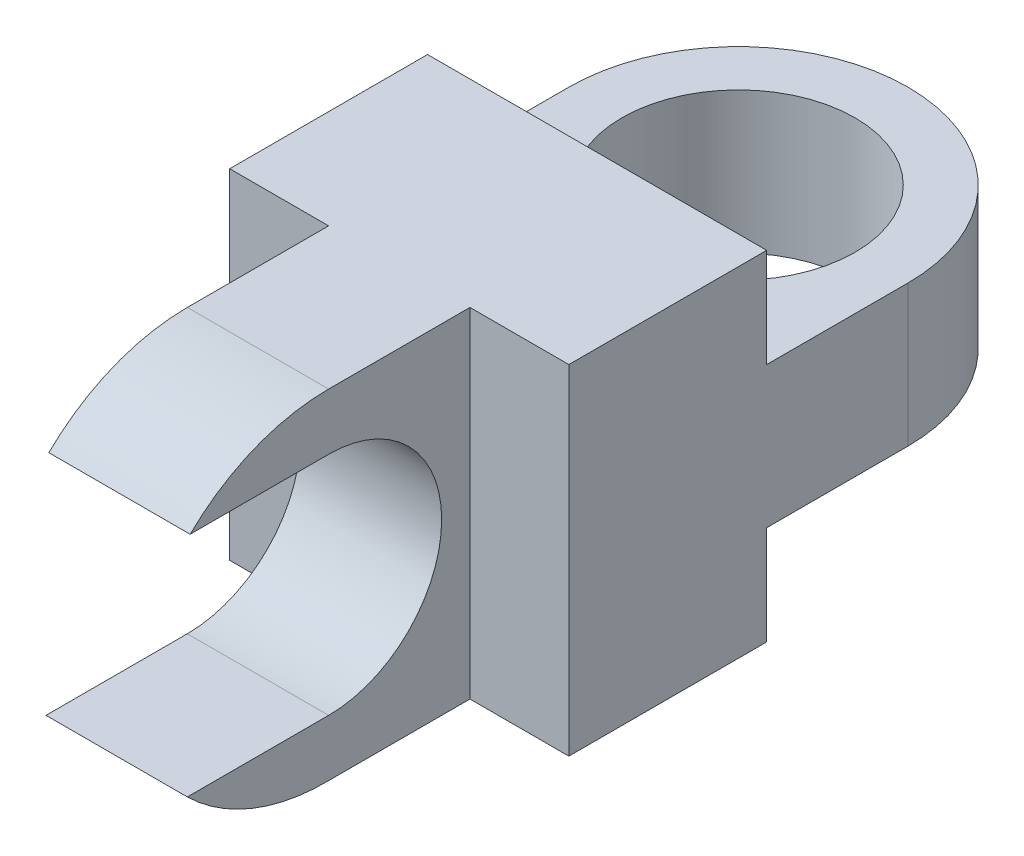
ISO-10303-21;
HEADER;
FILE_DESCRIPTION(('STEP AP214'),'2;1');
FILE_NAME('part.step','',(''),(''),'','','');
FILE_SCHEMA(('AUTOMOTIVE_DESIGN { 1 0 10303 214 1 1 1 1 }'));
ENDSEC;
DATA;
#1=APPLICATION_CONTEXT('core data for automotive mechanical design processes');
#2=APPLICATION_PROTOCOL_DEFINITION('international standard','automotive_design',2000,#1);
#3=PRODUCT_CONTEXT('',#1,'mechanical');
#4=PRODUCT('Part','Part','',(#3));
#5=PRODUCT_RELATED_PRODUCT_CATEGORY('part','',(#4));
#6=PRODUCT_DEFINITION_FORMATION('','',#4);
#7=PRODUCT_DEFINITION_CONTEXT('part definition',#1,'design');
#8=PRODUCT_DEFINITION('design','',#6,#7);
#9=PRODUCT_DEFINITION_SHAPE('','',#8);
#10=(LENGTH_UNIT() NAMED_UNIT(*) SI_UNIT(.MILLI.,.METRE.));
#11=(NAMED_UNIT(*) PLANE_ANGLE_UNIT() SI_UNIT($,.RADIAN.));
#12=(NAMED_UNIT(*) SI_UNIT($,.STERADIAN.) SOLID_ANGLE_UNIT());
#13=UNCERTAINTY_MEASURE_WITH_UNIT(LENGTH_MEASURE(1.E-05),#10,'distance_accuracy_value','');
#14=(GEOMETRIC_REPRESENTATION_CONTEXT(3) GLOBAL_UNCERTAINTY_ASSIGNED_CONTEXT((#13)) GLOBAL_UNIT_ASSIGNED_CONTEXT((#10,
#11,#12)) REPRESENTATION_CONTEXT('',''));
#15=CARTESIAN_POINT('',(0.,0.,0.));
#16=DIRECTION('',(0.,0.,1.));
#17=DIRECTION('',(1.,0.,0.));
#18=AXIS2_PLACEMENT_3D('',#15,#16,#17);
#19=CARTESIAN_POINT('',(0.,0.,0.));
#20=DIRECTION('',(0.,0.,-1.));
#21=DIRECTION('',(-1.,0.,0.));
#22=AXIS2_PLACEMENT_3D('',#19,#20,#21);
#23=PLANE('',#22);
#24=DIRECTION('',(0.,-1.,0.));
#25=VECTOR('',#24,1.);
#26=CARTESIAN_POINT('',(0.,-48.,0.));
#27=LINE('',#26,#25);
#28=CARTESIAN_POINT('',(0.,-34.,0.));
#29=VERTEX_POINT('',#28);
#30=CARTESIAN_POINT('',(0.,-48.,0.));
#31=VERTEX_POINT('',#30);
#32=EDGE_CURVE('E277',#29,#31,#27,.T.);
#33=ORIENTED_EDGE('',*,*,#32,.F.);
#34=DIRECTION('',(1.,0.,0.));
#35=VECTOR('',#34,1.);
#36=CARTESIAN_POINT('',(0.,-34.,0.));
#37=LINE('',#36,#35);
#38=CARTESIAN_POINT('',(48.,-34.,0.));
#39=VERTEX_POINT('',#38);
#40=EDGE_CURVE('E248',#29,#39,#37,.T.);
#41=ORIENTED_EDGE('',*,*,#40,.T.);
#42=DIRECTION('',(0.,1.,0.));
#43=VECTOR('',#42,1.);
#44=CARTESIAN_POINT('',(48.,0.,0.));
#45=LINE('',#44,#43);
#46=CARTESIAN_POINT('',(48.,-48.,0.));
#47=VERTEX_POINT('',#46);
#48=EDGE_CURVE('E299',#47,#39,#45,.T.);
#49=ORIENTED_EDGE('',*,*,#48,.F.);
#50=DIRECTION('',(1.,0.,0.));
#51=VECTOR('',#50,1.);
#52=CARTESIAN_POINT('',(48.,-48.,0.));
#53=LINE('',#52,#51);
#54=EDGE_CURVE('E298',#31,#47,#53,.T.);
#55=ORIENTED_EDGE('',*,*,#54,.F.);
#56=EDGE_LOOP('',(#33,#41,#49,#55));
#57=FACE_BOUND('',#56,.T.);
#58=ADVANCED_FACE('F50',(#57),#23,.T.);
#59=CARTESIAN_POINT('',(0.,0.,28.));
#60=DIRECTION('',(0.,0.,-1.));
#61=DIRECTION('',(-1.,0.,0.));
#62=AXIS2_PLACEMENT_3D('',#59,#60,#61);
#63=PLANE('',#62);
#64=DIRECTION('',(0.,1.,0.));
#65=VECTOR('',#64,1.);
#66=CARTESIAN_POINT('',(34.,-48.,28.));
#67=LINE('',#66,#65);
#68=CARTESIAN_POINT('',(34.,-48.,28.));
#69=VERTEX_POINT('',#68);
#70=CARTESIAN_POINT('',(34.,0.,28.));
#71=VERTEX_POINT('',#70);
#72=EDGE_CURVE('E269',#69,#71,#67,.T.);
#73=ORIENTED_EDGE('',*,*,#72,.F.);
#74=DIRECTION('',(1.,0.,0.));
#75=VECTOR('',#74,1.);
#76=CARTESIAN_POINT('',(48.,-48.,28.));
#77=LINE('',#76,#75);
#78=CARTESIAN_POINT('',(48.,-48.,28.));
#79=VERTEX_POINT('',#78);
#80=EDGE_CURVE('E284',#69,#79,#77,.T.);
#81=ORIENTED_EDGE('',*,*,#80,.T.);
#82=DIRECTION('',(0.,1.,0.));
#83=VECTOR('',#82,1.);
#84=CARTESIAN_POINT('',(48.,0.,28.));
#85=LINE('',#84,#83);
#86=CARTESIAN_POINT('',(48.,0.,28.));
#87=VERTEX_POINT('',#86);
#88=EDGE_CURVE('E287',#79,#87,#85,.T.);
#89=ORIENTED_EDGE('',*,*,#88,.T.);
#90=DIRECTION('',(-1.,0.,0.));
#91=VECTOR('',#90,1.);
#92=CARTESIAN_POINT('',(0.,0.,28.));
#93=LINE('',#92,#91);
#94=EDGE_CURVE('E286',#87,#71,#93,.T.);
#95=ORIENTED_EDGE('',*,*,#94,.T.);
#96=EDGE_LOOP('',(#73,#81,#89,#95));
#97=FACE_BOUND('',#96,.T.);
#98=ADVANCED_FACE('F359',(#97),#63,.F.);
#99=CARTESIAN_POINT('',(0.,-48.,28.));
#100=DIRECTION('',(1.,0.,0.));
#101=DIRECTION('',(0.,0.,-1.));
#102=AXIS2_PLACEMENT_3D('',#99,#100,#101);
#103=PLANE('',#102);
#104=CARTESIAN_POINT('',(0.,0.,0.));
#105=VERTEX_POINT('',#104);
#106=CARTESIAN_POINT('',(0.,-14.,0.));
#107=VERTEX_POINT('',#106);
#108=EDGE_CURVE('E291',#105,#107,#27,.T.);
#109=ORIENTED_EDGE('',*,*,#108,.T.);
#110=DIRECTION('',(0.,0.,1.));
#111=VECTOR('',#110,1.);
#112=CARTESIAN_POINT('',(0.,-14.,-20.));
#113=LINE('',#112,#111);
#114=CARTESIAN_POINT('',(0.,-14.,-20.));
#115=VERTEX_POINT('',#114);
#116=EDGE_CURVE('E250',#115,#107,#113,.T.);
#117=ORIENTED_EDGE('',*,*,#116,.F.);
#118=DIRECTION('',(0.,1.,0.));
#119=VECTOR('',#118,1.);
#120=CARTESIAN_POINT('',(0.,-34.,-20.));
#121=LINE('',#120,#119);
#122=CARTESIAN_POINT('',(0.,-34.,-20.));
#123=VERTEX_POINT('',#122);
#124=EDGE_CURVE('E242',#123,#115,#121,.T.);
#125=ORIENTED_EDGE('',*,*,#124,.F.);
#126=DIRECTION('',(0.,0.,-1.));
#127=VECTOR('',#126,1.);
#128=CARTESIAN_POINT('',(0.,-34.,0.));
#129=LINE('',#128,#127);
#130=EDGE_CURVE('E241',#29,#123,#129,.T.);
#131=ORIENTED_EDGE('',*,*,#130,.F.);
#132=ORIENTED_EDGE('',*,*,#32,.T.);
#133=DIRECTION('',(0.,0.,-1.));
#134=VECTOR('',#133,1.);
#135=CARTESIAN_POINT('',(0.,-48.,28.));
#136=LINE('',#135,#134);
#137=CARTESIAN_POINT('',(0.,-48.,28.));
#138=VERTEX_POINT('',#137);
#139=EDGE_CURVE('E11',#138,#31,#136,.T.);
#140=ORIENTED_EDGE('',*,*,#139,.F.);
#141=DIRECTION('',(0.,-1.,0.));
#142=VECTOR('',#141,1.);
#143=CARTESIAN_POINT('',(0.,-48.,28.));
#144=LINE('',#143,#142);
#145=CARTESIAN_POINT('',(0.,0.,28.));
#146=VERTEX_POINT('',#145);
#147=EDGE_CURVE('E279',#146,#138,#144,.T.);
#148=ORIENTED_EDGE('',*,*,#147,.F.);
#149=DIRECTION('',(0.,0.,-1.));
#150=VECTOR('',#149,1.);
#151=CARTESIAN_POINT('',(0.,0.,28.));
#152=LINE('',#151,#150);
#153=EDGE_CURVE('E292',#146,#105,#152,.T.);
#154=ORIENTED_EDGE('',*,*,#153,.T.);
#155=EDGE_LOOP('',(#109,#117,#125,#131,#132,#140,#148,#154));
#156=FACE_BOUND('',#155,.T.);
#157=ADVANCED_FACE('F47',(#156),#103,.F.);
#158=CARTESIAN_POINT('',(48.,-48.,28.));
#159=DIRECTION('',(0.,1.,0.));
#160=DIRECTION('',(0.,0.,1.));
#161=AXIS2_PLACEMENT_3D('',#158,#159,#160);
#162=PLANE('',#161);
#163=ORIENTED_EDGE('',*,*,#54,.T.);
#164=DIRECTION('',(0.,0.,-1.));
#165=VECTOR('',#164,1.);
#166=CARTESIAN_POINT('',(48.,-48.,28.));
#167=LINE('',#166,#165);
#168=EDGE_CURVE('E54',#79,#47,#167,.T.);
#169=ORIENTED_EDGE('',*,*,#168,.F.);
#170=ORIENTED_EDGE('',*,*,#80,.F.);
#171=DIRECTION('',(0.,0.,1.));
#172=VECTOR('',#171,1.);
#173=CARTESIAN_POINT('',(34.,-48.,0.));
#174=LINE('',#173,#172);
#175=CARTESIAN_POINT('',(34.,-48.,48.));
#176=VERTEX_POINT('',#175);
#177=EDGE_CURVE('E262',#69,#176,#174,.T.);
#178=ORIENTED_EDGE('',*,*,#177,.T.);
#179=DIRECTION('',(-1.,0.,0.));
#180=VECTOR('',#179,1.);
#181=CARTESIAN_POINT('',(0.,-48.,48.));
#182=LINE('',#181,#180);
#183=CARTESIAN_POINT('',(14.,-48.,48.));
#184=VERTEX_POINT('',#183);
#185=EDGE_CURVE('E261',#176,#184,#182,.T.);
#186=ORIENTED_EDGE('',*,*,#185,.T.);
#187=DIRECTION('',(0.,0.,-1.));
#188=VECTOR('',#187,1.);
#189=CARTESIAN_POINT('',(14.,-48.,0.));
#190=LINE('',#189,#188);
#191=CARTESIAN_POINT('',(14.,-48.,28.));
#192=VERTEX_POINT('',#191);
#193=EDGE_CURVE('E258',#184,#192,#190,.T.);
#194=ORIENTED_EDGE('',*,*,#193,.T.);
#195=EDGE_CURVE('E285',#138,#192,#77,.T.);
#196=ORIENTED_EDGE('',*,*,#195,.F.);
#197=ORIENTED_EDGE('',*,*,#139,.T.);
#198=EDGE_LOOP('',(#163,#169,#170,#178,#186,#194,#196,#197));
#199=FACE_BOUND('',#198,.T.);
#200=ADVANCED_FACE('F363',(#199),#162,.F.);
#201=CARTESIAN_POINT('',(48.,0.,28.));
#202=DIRECTION('',(-1.,0.,0.));
#203=DIRECTION('',(0.,0.,1.));
#204=AXIS2_PLACEMENT_3D('',#201,#202,#203);
#205=PLANE('',#204);
#206=ORIENTED_EDGE('',*,*,#48,.T.);
#207=DIRECTION('',(0.,0.,-1.));
#208=VECTOR('',#207,1.);
#209=CARTESIAN_POINT('',(48.,-34.,0.));
#210=LINE('',#209,#208);
#211=CARTESIAN_POINT('',(48.,-34.,-20.));
#212=VERTEX_POINT('',#211);
#213=EDGE_CURVE('E67',#39,#212,#210,.T.);
#214=ORIENTED_EDGE('',*,*,#213,.T.);
#215=DIRECTION('',(0.,1.,0.));
#216=VECTOR('',#215,1.);
#217=CARTESIAN_POINT('',(48.,-34.,-20.));
#218=LINE('',#217,#216);
#219=CARTESIAN_POINT('',(48.,-14.,-20.));
#220=VERTEX_POINT('',#219);
#221=EDGE_CURVE('E252',#212,#220,#218,.T.);
#222=ORIENTED_EDGE('',*,*,#221,.T.);
#223=DIRECTION('',(0.,0.,1.));
#224=VECTOR('',#223,1.);
#225=CARTESIAN_POINT('',(48.,-14.,-20.));
#226=LINE('',#225,#224);
#227=CARTESIAN_POINT('',(48.,-14.,0.));
#228=VERTEX_POINT('',#227);
#229=EDGE_CURVE('E244',#220,#228,#226,.T.);
#230=ORIENTED_EDGE('',*,*,#229,.T.);
#231=CARTESIAN_POINT('',(48.,0.,0.));
#232=VERTEX_POINT('',#231);
#233=EDGE_CURVE('E296',#228,#232,#45,.T.);
#234=ORIENTED_EDGE('',*,*,#233,.T.);
#235=DIRECTION('',(0.,0.,-1.));
#236=VECTOR('',#235,1.);
#237=CARTESIAN_POINT('',(48.,0.,28.));
#238=LINE('',#237,#236);
#239=EDGE_CURVE('E304',#87,#232,#238,.T.);
#240=ORIENTED_EDGE('',*,*,#239,.F.);
#241=ORIENTED_EDGE('',*,*,#88,.F.);
#242=ORIENTED_EDGE('',*,*,#168,.T.);
#243=EDGE_LOOP('',(#206,#214,#222,#230,#234,#240,#241,#242));
#244=FACE_BOUND('',#243,.T.);
#245=ADVANCED_FACE('F315',(#244),#205,.F.);
#246=CARTESIAN_POINT('',(0.,0.,28.));
#247=DIRECTION('',(0.,-1.,0.));
#248=DIRECTION('',(0.,0.,-1.));
#249=AXIS2_PLACEMENT_3D('',#246,#247,#248);
#250=PLANE('',#249);
#251=DIRECTION('',(-1.,0.,0.));
#252=VECTOR('',#251,1.);
#253=CARTESIAN_POINT('',(0.,0.,0.));
#254=LINE('',#253,#252);
#255=EDGE_CURVE('E281',#232,#105,#254,.T.);
#256=ORIENTED_EDGE('',*,*,#255,.T.);
#257=ORIENTED_EDGE('',*,*,#153,.F.);
#258=CARTESIAN_POINT('',(14.,0.,28.));
#259=VERTEX_POINT('',#258);
#260=EDGE_CURVE('E290',#259,#146,#93,.T.);
#261=ORIENTED_EDGE('',*,*,#260,.F.);
#262=DIRECTION('',(0.,0.,-1.));
#263=VECTOR('',#262,1.);
#264=CARTESIAN_POINT('',(14.,0.,0.));
#265=LINE('',#264,#263);
#266=CARTESIAN_POINT('',(14.,0.,48.));
#267=VERTEX_POINT('',#266);
#268=EDGE_CURVE('E259',#267,#259,#265,.T.);
#269=ORIENTED_EDGE('',*,*,#268,.F.);
#270=DIRECTION('',(-1.,0.,0.));
#271=VECTOR('',#270,1.);
#272=CARTESIAN_POINT('',(0.,0.,48.));
#273=LINE('',#272,#271);
#274=CARTESIAN_POINT('',(34.,0.,48.));
#275=VERTEX_POINT('',#274);
#276=EDGE_CURVE('E266',#275,#267,#273,.T.);
#277=ORIENTED_EDGE('',*,*,#276,.F.);
#278=DIRECTION('',(0.,0.,1.));
#279=VECTOR('',#278,1.);
#280=CARTESIAN_POINT('',(34.,0.,0.));
#281=LINE('',#280,#279);
#282=EDGE_CURVE('E265',#71,#275,#281,.T.);
#283=ORIENTED_EDGE('',*,*,#282,.F.);
#284=ORIENTED_EDGE('',*,*,#94,.F.);
#285=ORIENTED_EDGE('',*,*,#239,.T.);
#286=EDGE_LOOP('',(#256,#257,#261,#269,#277,#283,#284,#285));
#287=FACE_BOUND('',#286,.T.);
#288=ADVANCED_FACE('F339',(#287),#250,.F.);
#289=ORIENTED_EDGE('',*,*,#195,.T.);
#290=DIRECTION('',(0.,1.,0.));
#291=VECTOR('',#290,1.);
#292=CARTESIAN_POINT('',(14.,-48.,28.));
#293=LINE('',#292,#291);
#294=EDGE_CURVE('E271',#192,#259,#293,.T.);
#295=ORIENTED_EDGE('',*,*,#294,.T.);
#296=ORIENTED_EDGE('',*,*,#260,.T.);
#297=ORIENTED_EDGE('',*,*,#147,.T.);
#298=EDGE_LOOP('',(#289,#295,#296,#297));
#299=FACE_BOUND('',#298,.T.);
#300=ADVANCED_FACE('F341',(#299),#63,.F.);
#301=DIRECTION('',(1.,0.,0.));
#302=VECTOR('',#301,1.);
#303=CARTESIAN_POINT('',(0.,-14.,0.));
#304=LINE('',#303,#302);
#305=EDGE_CURVE('E257',#107,#228,#304,.T.);
#306=ORIENTED_EDGE('',*,*,#305,.F.);
#307=ORIENTED_EDGE('',*,*,#108,.F.);
#308=ORIENTED_EDGE('',*,*,#255,.F.);
#309=ORIENTED_EDGE('',*,*,#233,.F.);
#310=EDGE_LOOP('',(#306,#307,#308,#309));
#311=FACE_BOUND('',#310,.T.);
#312=ADVANCED_FACE('F333',(#311),#23,.T.);
#313=CARTESIAN_POINT('',(14.,-48.,0.));
#314=DIRECTION('',(1.,0.,0.));
#315=DIRECTION('',(0.,0.,-1.));
#316=AXIS2_PLACEMENT_3D('',#313,#314,#315);
#317=PLANE('',#316);
#318=CARTESIAN_POINT('',(14.,-24.,48.));
#319=DIRECTION('',(1.,0.,0.));
#320=DIRECTION('',(0.,0.,-1.));
#321=AXIS2_PLACEMENT_3D('',#318,#319,#320);
#322=CIRCLE('',#321,16.);
#323=CARTESIAN_POINT('',(14.,-40.,48.));
#324=VERTEX_POINT('',#323);
#325=CARTESIAN_POINT('',(14.,-7.99999999999999,48.));
#326=VERTEX_POINT('',#325);
#327=EDGE_CURVE('E177',#324,#326,#322,.T.);
#328=ORIENTED_EDGE('',*,*,#327,.T.);
#329=DIRECTION('',(0.,-1.,0.));
#330=VECTOR('',#329,1.);
#331=CARTESIAN_POINT('',(14.,0.,48.));
#332=LINE('',#331,#330);
#333=CARTESIAN_POINT('',(14.,-8.00287373526744,48.));
#334=VERTEX_POINT('',#333);
#335=EDGE_CURVE('E187',#326,#334,#332,.T.);
#336=ORIENTED_EDGE('',*,*,#335,.T.);
#337=DIRECTION('',(0.,0.,1.));
#338=VECTOR('',#337,1.);
#339=CARTESIAN_POINT('',(14.,-8.00287373526742,0.));
#340=LINE('',#339,#338);
#341=CARTESIAN_POINT('',(14.,-8.00287373526744,67.598850505893));
#342=VERTEX_POINT('',#341);
#343=EDGE_CURVE('E220',#334,#342,#340,.T.);
#344=ORIENTED_EDGE('',*,*,#343,.T.);
#345=CARTESIAN_POINT('',(14.,-28.,48.));
#346=DIRECTION('',(1.,0.,0.));
#347=DIRECTION('',(0.,0.,-1.));
#348=AXIS2_PLACEMENT_3D('',#345,#346,#347);
#349=CIRCLE('',#348,28.);
#350=EDGE_CURVE('E213',#342,#267,#349,.F.);
#351=ORIENTED_EDGE('',*,*,#350,.T.);
#352=ORIENTED_EDGE('',*,*,#268,.T.);
#353=ORIENTED_EDGE('',*,*,#294,.F.);
#354=ORIENTED_EDGE('',*,*,#193,.F.);
#355=CARTESIAN_POINT('',(14.,-20.0028324812059,48.3982598706638));
#356=DIRECTION('',(1.,0.,0.));
#357=DIRECTION('',(0.,0.,-1.));
#358=AXIS2_PLACEMENT_3D('',#355,#356,#357);
#359=CIRCLE('',#358,28.);
#360=CARTESIAN_POINT('',(14.,-39.9971262647326,68.));
#361=VERTEX_POINT('',#360);
#362=EDGE_CURVE('E204',#361,#184,#359,.T.);
#363=ORIENTED_EDGE('',*,*,#362,.F.);
#364=DIRECTION('',(0.,0.,1.));
#365=VECTOR('',#364,1.);
#366=CARTESIAN_POINT('',(14.,-39.9971262647326,0.));
#367=LINE('',#366,#365);
#368=CARTESIAN_POINT('',(14.,-39.9971262647326,48.));
#369=VERTEX_POINT('',#368);
#370=EDGE_CURVE('E195',#369,#361,#367,.T.);
#371=ORIENTED_EDGE('',*,*,#370,.F.);
#372=EDGE_CURVE('E65',#369,#324,#332,.T.);
#373=ORIENTED_EDGE('',*,*,#372,.T.);
#374=EDGE_LOOP('',(#328,#336,#344,#351,#352,#353,#354,#363,#371,#373));
#375=FACE_BOUND('',#374,.T.);
#376=ADVANCED_FACE('F186',(#375),#317,.F.);
#377=CARTESIAN_POINT('',(34.,-48.,0.));
#378=DIRECTION('',(-1.,0.,0.));
#379=DIRECTION('',(0.,0.,1.));
#380=AXIS2_PLACEMENT_3D('',#377,#378,#379);
#381=PLANE('',#380);
#382=CARTESIAN_POINT('',(34.,-24.,48.));
#383=DIRECTION('',(1.,0.,0.));
#384=DIRECTION('',(0.,0.,-1.));
#385=AXIS2_PLACEMENT_3D('',#382,#383,#384);
#386=CIRCLE('',#385,16.);
#387=CARTESIAN_POINT('',(34.,-40.,48.));
#388=VERTEX_POINT('',#387);
#389=CARTESIAN_POINT('',(34.,-7.99999999999999,48.));
#390=VERTEX_POINT('',#389);
#391=EDGE_CURVE('E194',#388,#390,#386,.T.);
#392=ORIENTED_EDGE('',*,*,#391,.F.);
#393=DIRECTION('',(0.,-1.,0.));
#394=VECTOR('',#393,1.);
#395=CARTESIAN_POINT('',(34.,0.,48.));
#396=LINE('',#395,#394);
#397=CARTESIAN_POINT('',(34.,-39.9971262647326,48.));
#398=VERTEX_POINT('',#397);
#399=EDGE_CURVE('E172',#398,#388,#396,.T.);
#400=ORIENTED_EDGE('',*,*,#399,.F.);
#401=DIRECTION('',(0.,0.,1.));
#402=VECTOR('',#401,1.);
#403=CARTESIAN_POINT('',(34.,-39.9971262647326,0.));
#404=LINE('',#403,#402);
#405=CARTESIAN_POINT('',(34.,-39.9971262647326,68.));
#406=VERTEX_POINT('',#405);
#407=EDGE_CURVE('E198',#398,#406,#404,.T.);
#408=ORIENTED_EDGE('',*,*,#407,.T.);
#409=CARTESIAN_POINT('',(34.,-20.0028324812059,48.3982598706638));
#410=DIRECTION('',(1.,0.,0.));
#411=DIRECTION('',(0.,0.,-1.));
#412=AXIS2_PLACEMENT_3D('',#409,#410,#411);
#413=CIRCLE('',#412,28.);
#414=EDGE_CURVE('E205',#406,#176,#413,.T.);
#415=ORIENTED_EDGE('',*,*,#414,.T.);
#416=ORIENTED_EDGE('',*,*,#177,.F.);
#417=ORIENTED_EDGE('',*,*,#72,.T.);
#418=ORIENTED_EDGE('',*,*,#282,.T.);
#419=CARTESIAN_POINT('',(34.,-28.,48.));
#420=DIRECTION('',(1.,0.,0.));
#421=DIRECTION('',(0.,0.,-1.));
#422=AXIS2_PLACEMENT_3D('',#419,#420,#421);
#423=CIRCLE('',#422,28.);
#424=CARTESIAN_POINT('',(34.,-8.00287373526744,67.598850505893));
#425=VERTEX_POINT('',#424);
#426=EDGE_CURVE('E214',#425,#275,#423,.F.);
#427=ORIENTED_EDGE('',*,*,#426,.F.);
#428=DIRECTION('',(0.,0.,1.));
#429=VECTOR('',#428,1.);
#430=CARTESIAN_POINT('',(34.,-8.00287373526742,0.));
#431=LINE('',#430,#429);
#432=CARTESIAN_POINT('',(34.,-8.00287373526744,48.));
#433=VERTEX_POINT('',#432);
#434=EDGE_CURVE('E218',#433,#425,#431,.T.);
#435=ORIENTED_EDGE('',*,*,#434,.F.);
#436=EDGE_CURVE('E193',#390,#433,#396,.T.);
#437=ORIENTED_EDGE('',*,*,#436,.F.);
#438=EDGE_LOOP('',(#392,#400,#408,#415,#416,#417,#418,#427,#435,#437));
#439=FACE_BOUND('',#438,.T.);
#440=ADVANCED_FACE('F358',(#439),#381,.F.);
#441=CARTESIAN_POINT('',(0.,-14.,-20.));
#442=DIRECTION('',(0.,1.,0.));
#443=DIRECTION('',(0.,0.,1.));
#444=AXIS2_PLACEMENT_3D('',#441,#442,#443);
#445=PLANE('',#444);
#446=CARTESIAN_POINT('',(24.,-14.,-20.));
#447=DIRECTION('',(0.,1.,0.));
#448=DIRECTION('',(0.,0.,1.));
#449=AXIS2_PLACEMENT_3D('',#446,#447,#448);
#450=CIRCLE('',#449,16.5);
#451=CARTESIAN_POINT('',(24.,-14.,-3.5));
#452=VERTEX_POINT('',#451);
#453=EDGE_CURVE('E226',#452,#452,#450,.T.);
#454=ORIENTED_EDGE('',*,*,#453,.F.);
#455=EDGE_LOOP('',(#454));
#456=FACE_BOUND('',#455,.T.);
#457=ORIENTED_EDGE('',*,*,#229,.F.);
#458=CARTESIAN_POINT('',(24.,-14.,-20.));
#459=DIRECTION('',(0.,1.,0.));
#460=DIRECTION('',(0.,0.,1.));
#461=AXIS2_PLACEMENT_3D('',#458,#459,#460);
#462=CIRCLE('',#461,24.);
#463=EDGE_CURVE('E234',#220,#115,#462,.T.);
#464=ORIENTED_EDGE('',*,*,#463,.T.);
#465=ORIENTED_EDGE('',*,*,#116,.T.);
#466=ORIENTED_EDGE('',*,*,#305,.T.);
#467=EDGE_LOOP('',(#457,#464,#465,#466));
#468=FACE_BOUND('',#467,.T.);
#469=ADVANCED_FACE('F327',(#456,#468),#445,.T.);
#470=CARTESIAN_POINT('',(0.,-34.,0.));
#471=DIRECTION('',(0.,-1.,0.));
#472=DIRECTION('',(0.,0.,-1.));
#473=AXIS2_PLACEMENT_3D('',#470,#471,#472);
#474=PLANE('',#473);
#475=CARTESIAN_POINT('',(24.,-34.,-20.));
#476=DIRECTION('',(0.,1.,0.));
#477=DIRECTION('',(0.,0.,1.));
#478=AXIS2_PLACEMENT_3D('',#475,#476,#477);
#479=CIRCLE('',#478,16.5);
#480=CARTESIAN_POINT('',(24.,-34.,-3.5));
#481=VERTEX_POINT('',#480);
#482=EDGE_CURVE('E233',#481,#481,#479,.T.);
#483=ORIENTED_EDGE('',*,*,#482,.T.);
#484=EDGE_LOOP('',(#483));
#485=FACE_BOUND('',#484,.T.);
#486=ORIENTED_EDGE('',*,*,#213,.F.);
#487=ORIENTED_EDGE('',*,*,#40,.F.);
#488=ORIENTED_EDGE('',*,*,#130,.T.);
#489=CARTESIAN_POINT('',(24.,-34.,-20.));
#490=DIRECTION('',(0.,1.,0.));
#491=DIRECTION('',(0.,0.,1.));
#492=AXIS2_PLACEMENT_3D('',#489,#490,#491);
#493=CIRCLE('',#492,24.);
#494=EDGE_CURVE('E240',#212,#123,#493,.T.);
#495=ORIENTED_EDGE('',*,*,#494,.F.);
#496=EDGE_LOOP('',(#486,#487,#488,#495));
#497=FACE_BOUND('',#496,.T.);
#498=ADVANCED_FACE('F318',(#485,#497),#474,.T.);
#499=CARTESIAN_POINT('',(24.,-34.,-20.));
#500=DIRECTION('',(0.,1.,0.));
#501=DIRECTION('',(0.,0.,1.));
#502=AXIS2_PLACEMENT_3D('',#499,#500,#501);
#503=CYLINDRICAL_SURFACE('',#502,24.);
#504=ORIENTED_EDGE('',*,*,#463,.F.);
#505=ORIENTED_EDGE('',*,*,#221,.F.);
#506=ORIENTED_EDGE('',*,*,#494,.T.);
#507=ORIENTED_EDGE('',*,*,#124,.T.);
#508=EDGE_LOOP('',(#504,#505,#506,#507));
#509=FACE_BOUND('',#508,.T.);
#510=ADVANCED_FACE('F329',(#509),#503,.T.);
#511=CARTESIAN_POINT('',(24.,-34.,-20.));
#512=DIRECTION('',(0.,1.,0.));
#513=DIRECTION('',(0.,0.,1.));
#514=AXIS2_PLACEMENT_3D('',#511,#512,#513);
#515=CYLINDRICAL_SURFACE('',#514,16.5);
#516=ORIENTED_EDGE('',*,*,#482,.F.);
#517=EDGE_LOOP('',(#516));
#518=FACE_BOUND('',#517,.T.);
#519=ORIENTED_EDGE('',*,*,#453,.T.);
#520=EDGE_LOOP('',(#519));
#521=FACE_BOUND('',#520,.T.);
#522=ADVANCED_FACE('F408',(#518,#521),#515,.F.);
#523=CARTESIAN_POINT('',(14.,-28.,48.));
#524=DIRECTION('',(1.,0.,0.));
#525=DIRECTION('',(0.,0.,-1.));
#526=AXIS2_PLACEMENT_3D('',#523,#524,#525);
#527=CYLINDRICAL_SURFACE('',#526,28.);
#528=ORIENTED_EDGE('',*,*,#426,.T.);
#529=ORIENTED_EDGE('',*,*,#276,.T.);
#530=ORIENTED_EDGE('',*,*,#350,.F.);
#531=DIRECTION('',(1.,0.,0.));
#532=VECTOR('',#531,1.);
#533=CARTESIAN_POINT('',(14.,-8.00287373526744,67.598850505893));
#534=LINE('',#533,#532);
#535=EDGE_CURVE('E222',#342,#425,#534,.T.);
#536=ORIENTED_EDGE('',*,*,#535,.T.);
#537=EDGE_LOOP('',(#528,#529,#530,#536));
#538=FACE_BOUND('',#537,.T.);
#539=ADVANCED_FACE('F354',(#538),#527,.T.);
#540=CARTESIAN_POINT('',(14.,-8.00287373526742,0.));
#541=DIRECTION('',(0.,1.,0.));
#542=DIRECTION('',(0.,0.,1.));
#543=AXIS2_PLACEMENT_3D('',#540,#541,#542);
#544=PLANE('',#543);
#545=ORIENTED_EDGE('',*,*,#434,.T.);
#546=ORIENTED_EDGE('',*,*,#535,.F.);
#547=ORIENTED_EDGE('',*,*,#343,.F.);
#548=DIRECTION('',(1.,0.,0.));
#549=VECTOR('',#548,1.);
#550=CARTESIAN_POINT('',(14.,-8.00287373526744,48.));
#551=LINE('',#550,#549);
#552=EDGE_CURVE('E223',#334,#433,#551,.T.);
#553=ORIENTED_EDGE('',*,*,#552,.T.);
#554=EDGE_LOOP('',(#545,#546,#547,#553));
#555=FACE_BOUND('',#554,.T.);
#556=ADVANCED_FACE('F371',(#555),#544,.F.);
#557=CARTESIAN_POINT('',(14.,-39.9971262647326,0.));
#558=DIRECTION('',(0.,1.,0.));
#559=DIRECTION('',(0.,0.,1.));
#560=AXIS2_PLACEMENT_3D('',#557,#558,#559);
#561=PLANE('',#560);
#562=ORIENTED_EDGE('',*,*,#407,.F.);
#563=DIRECTION('',(1.,0.,0.));
#564=VECTOR('',#563,1.);
#565=CARTESIAN_POINT('',(14.,-39.9971262647326,48.));
#566=LINE('',#565,#564);
#567=EDGE_CURVE('E212',#369,#398,#566,.T.);
#568=ORIENTED_EDGE('',*,*,#567,.F.);
#569=ORIENTED_EDGE('',*,*,#370,.T.);
#570=DIRECTION('',(1.,0.,0.));
#571=VECTOR('',#570,1.);
#572=CARTESIAN_POINT('',(14.,-39.9971262647326,68.));
#573=LINE('',#572,#571);
#574=EDGE_CURVE('E207',#361,#406,#573,.T.);
#575=ORIENTED_EDGE('',*,*,#574,.T.);
#576=EDGE_LOOP('',(#562,#568,#569,#575));
#577=FACE_BOUND('',#576,.T.);
#578=ADVANCED_FACE('F367',(#577),#561,.T.);
#579=CARTESIAN_POINT('',(14.,-20.0028324812059,48.3982598706638));
#580=DIRECTION('',(1.,0.,0.));
#581=DIRECTION('',(0.,0.,-1.));
#582=AXIS2_PLACEMENT_3D('',#579,#580,#581);
#583=CYLINDRICAL_SURFACE('',#582,28.);
#584=ORIENTED_EDGE('',*,*,#414,.F.);
#585=ORIENTED_EDGE('',*,*,#574,.F.);
#586=ORIENTED_EDGE('',*,*,#362,.T.);
#587=ORIENTED_EDGE('',*,*,#185,.F.);
#588=EDGE_LOOP('',(#584,#585,#586,#587));
#589=FACE_BOUND('',#588,.T.);
#590=ADVANCED_FACE('F366',(#589),#583,.T.);
#591=CARTESIAN_POINT('',(14.,0.,48.));
#592=DIRECTION('',(0.,0.,1.));
#593=DIRECTION('',(0.,-1.,0.));
#594=AXIS2_PLACEMENT_3D('',#591,#592,#593);
#595=PLANE('',#594);
#596=ORIENTED_EDGE('',*,*,#335,.F.);
#597=DIRECTION('',(1.,0.,0.));
#598=VECTOR('',#597,1.);
#599=CARTESIAN_POINT('',(14.,-7.99999999999999,48.));
#600=LINE('',#599,#598);
#601=EDGE_CURVE('E178',#326,#390,#600,.T.);
#602=ORIENTED_EDGE('',*,*,#601,.T.);
#603=ORIENTED_EDGE('',*,*,#436,.T.);
#604=ORIENTED_EDGE('',*,*,#552,.F.);
#605=EDGE_LOOP('',(#596,#602,#603,#604));
#606=FACE_BOUND('',#605,.T.);
#607=ADVANCED_FACE('F377',(#606),#595,.F.);
#608=ORIENTED_EDGE('',*,*,#567,.T.);
#609=ORIENTED_EDGE('',*,*,#399,.T.);
#610=DIRECTION('',(1.,0.,0.));
#611=VECTOR('',#610,1.);
#612=CARTESIAN_POINT('',(14.,-40.,48.));
#613=LINE('',#612,#611);
#614=EDGE_CURVE('E167',#324,#388,#613,.T.);
#615=ORIENTED_EDGE('',*,*,#614,.F.);
#616=ORIENTED_EDGE('',*,*,#372,.F.);
#617=EDGE_LOOP('',(#608,#609,#615,#616));
#618=FACE_BOUND('',#617,.T.);
#619=ADVANCED_FACE('F175',(#618),#595,.F.);
#620=CARTESIAN_POINT('',(14.,-24.,48.));
#621=DIRECTION('',(1.,0.,0.));
#622=DIRECTION('',(0.,0.,-1.));
#623=AXIS2_PLACEMENT_3D('',#620,#621,#622);
#624=CYLINDRICAL_SURFACE('',#623,16.);
#625=ORIENTED_EDGE('',*,*,#391,.T.);
#626=ORIENTED_EDGE('',*,*,#601,.F.);
#627=ORIENTED_EDGE('',*,*,#327,.F.);
#628=ORIENTED_EDGE('',*,*,#614,.T.);
#629=EDGE_LOOP('',(#625,#626,#627,#628));
#630=FACE_BOUND('',#629,.T.);
#631=ADVANCED_FACE('F185',(#630),#624,.F.);
#632=CLOSED_SHELL('',(#58,#98,#157,#200,#245,#288,#300,#312,#376,#440,#469,#498,#510,#522,#539,
#556,#578,#590,#607,#619,#631));
#633=MANIFOLD_SOLID_BREP('B2',#632);
#634=ADVANCED_BREP_SHAPE_REPRESENTATION('',(#18,#633),#14);
#635=SHAPE_DEFINITION_REPRESENTATION(#9,#634);
ENDSEC;
END-ISO-10303-21;
